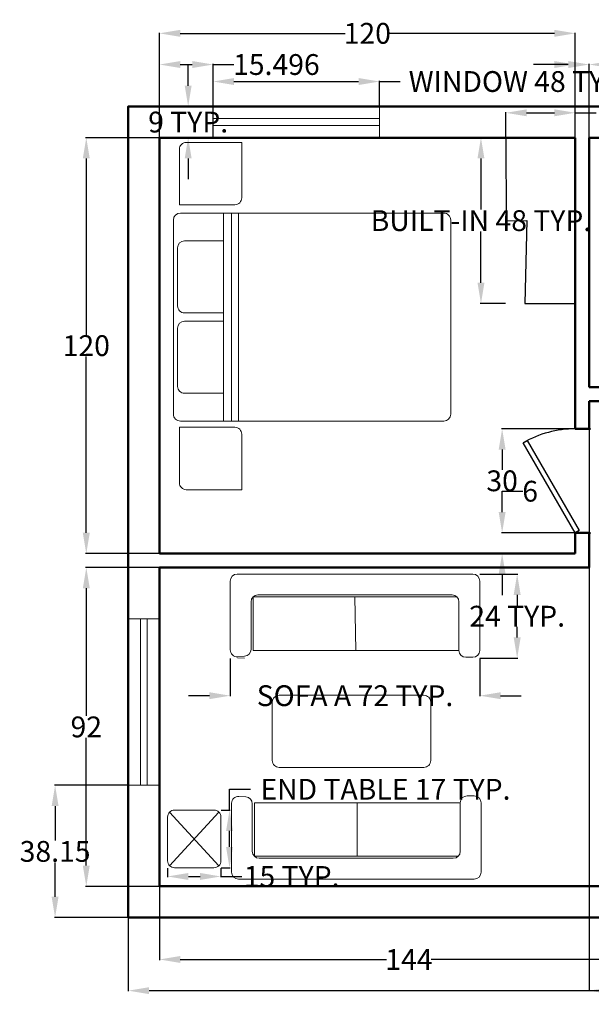
# Model space of a CAD drawing. Units: inches. Extents: x -22 to 471, y -231 to 53.
# Tile 1 of 3: x -22 to 143, y -231 to 53. Entities that reach past the tile are written whole.
import ezdxf

# ---------------------------------------------------------------- set-up
doc = ezdxf.new("R2010")
doc.units = ezdxf.units.IN
doc.header["$MEASUREMENT"] = 0
for name, color, linetype, lineweight in [('A-ANNO-DIMS', 2, 'Continuous', 18), ('A-DOOR', 3, 'Continuous', 25), ('A-FLOR-CASE', 32, 'Continuous', 25), ('A-FURN', 8, 'Continuous', 18), ('A-GLAZ', 4, 'Continuous', 18), ('A-WALL', 7, 'Continuous', 50)]:
    doc.layers.add(name, color=color, linetype=linetype, lineweight=lineweight)
doc.styles.get("Standard").update_dxf_attribs({"font": 'arial.ttf'})
doc.dimstyles.get("Standard").update_dxf_attribs({"dimtxt": 6, "dimasz": 6, "dimexe": 0.18, "dimexo": 0.0625, "dimgap": 0.09, "dimtad": 0, "dimtih": 1, "dimtoh": 1, "dimdec": 0, "dimzin": 0, "dimdsep": 46, "dimlunit": 4, "dimtxsty": 'Standard', "dimcen": 0.09, "dimadec": 0, "dimazin": 0, "dimtfac": 1, "dimtdec": 0, "dimtofl": 0, "dimtmove": 0, "dimatfit": 3, "dimfxl": 1, "dimtolj": 1, "dimtzin": 0, "dimarcsym": 0})

# ---------------------------------------------------------------- blocks, each defined once
blk = doc.blocks.new('Bed - Queen')
for p, q in [((2, 0), (58, 0)), ((0, -78), (0, -2)), ((10, -1.2), (26.8, -1.2)), ((33.2, -1.2), (50, -1.2)), ((60, -2), (60, -78)), ((8, -14.4), (8, -3.2)), ((28.8, -3.2), (28.8, -14.4)), ((31.2, -14.4), (31.2, -3.2)), ((52, -3.2), (52, -14.4)), ((0, -14.4), (60, -14.4)), ((60, -16.8), (0, -16.8)), ((60, -18.8), (0, -18.8)), ((58, -80), (2, -80))]:
    blk.add_line(p, q)
for points in [[(-17.8, -1.72), (-1.8, -1.72), (-1.8, -17.72, -0.414214), (-3.8, -19.72), (-19.8, -19.72), (-19.8, -3.72, -0.414214)], [(62.41, -1.72), (78.41, -1.72, -0.414214), (80.41, -3.72), (80.41, -19.72), (64.41, -19.72, -0.414214), (62.41, -17.72)]]:
    blk.add_lwpolyline(points, format="xyb", close=True)
for centre, start, end in [((2, -2), 90, 180), ((58, -2), 0, 90), ((10, -3.2), 90, 180), ((26.8, -3.2), 0, 90), ((33.2, -3.2), 90, 180), ((50, -3.2), 0, 90), ((2, -78), 180, 270), ((58, -78), 270, 0)]:
    blk.add_arc(centre, 2, start, end)
blk = doc.blocks.new('*U7')
for p, q in [((-40, 0), (-40, 6)), ((0, 0), (0, 6))]:
    blk.add_line(p, q)
blk.add_lwpolyline([(0, 0), (-34.64, -20), (-35.52, -18.48), (-0.87, 1.52)], close=True)
blk.add_arc((0, 0), 40, 180, 210)
blk = doc.blocks.new('WIN-48IN')
for p, q in [((0, 5.5), (48, 5.5)), ((0, 3.5), (48, 3.5))]:
    blk.add_line(p, q)
for points in [[(0, 0), (0, 9)], [(48, 9), (48, 0)]]:
    blk.add_lwpolyline(points)
blk = doc.blocks.new('SOFA-72IN-A')
for p, q in [((2, 24.28), (70, 24.28)), ((0, 2.42), (0, 22.28)), ((72, 22.28), (72, 2.28)), ((64, 18.28), (8, 18.28)), ((36.29, 2.28), (36, 17.7)), ((6, 16.28), (6, 2.56)), ((66, 2.28), (66, 16.28)), ((4.14, 0.57), (2.14, 0.43)), ((4.14, 0), (2.14, 0.14)), ((70, 0.28), (68, 0.28)), ((70, 0.28), (68, 0.28))]:
    blk.add_line(p, q)
blk.add_lwpolyline([(66, 16.28), (66, 2.28), (6.59, 2.28), (6.59, 17.7), (65.41, 17.7)])
for centre, start, end in [((2, 22.28), 90, 180), ((70, 22.28), 0, 90), ((8, 16.28), 90, 180), ((64, 16.28), 0, 90), ((2, 2.42), 180, 273.9184), ((4, 2.56), 273.9184, 0), ((68, 2.28), 180, 270), ((70, 2.28), 270, 0)]:
    blk.add_arc(centre, 2, start, end)
blk = doc.blocks.new('SOFA-72IN-B')
for p, q in [((2.14, 23.85), (4.14, 23.72)), ((68, 24), (70, 24)), ((0, 21.86), (0, 2)), ((6, 8), (6, 21.72)), ((36.29, 22), (36.29, 6.59)), ((66, 22), (66, 8)), ((72, 2), (72, 22)), ((64, 6), (8, 6)), ((2, 0), (70, 0))]:
    blk.add_line(p, q)
blk.add_lwpolyline([(66, 8), (66, 22), (6.59, 22), (6.59, 6.59), (65.41, 6.59)])
for centre, start, end in [((2, 21.86), 86.0816, 180), ((4, 21.72), 0, 86.0816), ((68, 22), 90, 180), ((70, 22), 0, 90), ((8, 8), 180, 270), ((64, 8), 270, 0), ((2, 2), 180, 270), ((70, 2), 270, 0)]:
    blk.add_arc(centre, 2, start, end)
blk = doc.blocks.new('TABLE-COFFEE')
blk.add_lwpolyline([(2, 20.83), (43.71, 20.83, -0.414214), (45.71, 18.83), (45.71, 2, -0.414214), (43.71, 0), (2, 0, -0.414214), (0, 2), (0, 18.83, -0.414214)], format="xyb", close=True)
blk = doc.blocks.new('TABLE-END')
for p, q in [((0.56, 0.61), (14.82, 16.04)), ((0.56, 16.04), (14.82, 0.61))]:
    blk.add_line(p, q)
blk.add_lwpolyline([(2, 16.65), (13.39, 16.65, -0.414214), (15.39, 14.65), (15.39, 2, -0.414214), (13.39, 0), (2, 0, -0.414214), (0, 2), (0, 14.65, -0.414214)], format="xyb", close=True)
blk = doc.blocks.new('BEDROOM-BUILTIN')
for p, q in [((0, 47.86), (0.1, 23.86)), ((0.1, 23.86), (6.1, 23.99)), ((6.1, 23.99), (5.51, 0)), ((5.51, 0), (20.03, 0))]:
    blk.add_line(p, q)
blk = doc.blocks.new('*D17')
at = {"layer": 'A-ANNO-DIMS', "color": 0, "lineweight": -2, "transparency": 16777216}
for p, q in [((33.43, 28.07), (33.43, 35.39)), ((39.43, 35.21), (75.43, 35.21)), ((81.43, 28.07), (81.43, 35.39)), ((81.43, 35.21), (87.43, 35.21))]:
    blk.add_line(p, q, dxfattribs=at)
at = {"layer": 'A-ANNO-DIMS', "color": 0, "transparency": 16777216}
for points in [[(39.43, 36.21), (39.43, 34.21), (33.43, 35.21)], [(75.43, 36.21), (75.43, 34.21), (81.43, 35.21)]]:
    blk.add_solid(points, dxfattribs=at)
at = {"layer": 'Defpoints', "color": 0, "transparency": 16777216}
for p in [(81.43, 35.21), (33.43, 28.01), (81.43, 28.01)]:
    blk.add_point(p, dxfattribs=at)
at = {"layer": 'A-ANNO-DIMS', "color": 0, "transparency": 16777216, "insert": (121.8, 35.21), "char_height": 6, "attachment_point": 5}
blk.add_mtext('\\A1;WINDOW 48 TYP.', dxfattribs=at)
blk = doc.blocks.new('*D18')
at = {"layer": 'A-ANNO-DIMS', "color": 0, "lineweight": -2, "transparency": 16777216}
for p, q in [((26.23, 34.01), (26.23, 40.01)), ((33.37, 28.01), (26.05, 28.01)), ((33.37, 19.01), (26.05, 19.01)), ((26.23, 13.01), (26.23, 7.01))]:
    blk.add_line(p, q, dxfattribs=at)
at = {"layer": 'A-ANNO-DIMS', "color": 0, "transparency": 16777216}
for points in [[(25.23, 34.01), (27.23, 34.01), (26.23, 28.01)], [(25.23, 13.01), (27.23, 13.01), (26.23, 19.01)]]:
    blk.add_solid(points, dxfattribs=at)
at = {"layer": 'Defpoints', "color": 0, "transparency": 16777216}
for p in [(26.23, 28.01), (33.43, 28.01), (33.43, 19.01)]:
    blk.add_point(p, dxfattribs=at)
at = {"layer": 'A-ANNO-DIMS', "color": 0, "transparency": 16777216, "insert": (26.23, 23.51), "char_height": 6, "attachment_point": 5}
blk.add_mtext('\\A1;9 TYP.', dxfattribs=at)
blk = doc.blocks.new('*D31')
at = {"layer": 'A-ANNO-DIMS', "color": 0, "lineweight": -2, "transparency": 16777216}
for p, q in [((38.37, -131.25), (38.37, -142.17)), ((110.37, -131.25), (110.37, -142.17)), ((32.37, -141.99), (26.37, -141.99)), ((116.37, -141.99), (122.37, -141.99))]:
    blk.add_line(p, q, dxfattribs=at)
at = {"layer": 'A-ANNO-DIMS', "color": 0, "transparency": 16777216}
for points in [[(32.37, -140.99), (32.37, -142.99), (38.37, -141.99)], [(116.37, -140.99), (116.37, -142.99), (110.37, -141.99)]]:
    blk.add_solid(points, dxfattribs=at)
at = {"layer": 'Defpoints', "color": 0, "transparency": 16777216}
for p in [(38.37, -131.19), (110.37, -131.19), (110.37, -141.99)]:
    blk.add_point(p, dxfattribs=at)
at = {"layer": 'A-ANNO-DIMS', "color": 0, "transparency": 16777216, "insert": (74.37, -141.99), "char_height": 6, "attachment_point": 5}
blk.add_mtext('\\A1;SOFA A 72 TYP.', dxfattribs=at)
blk = doc.blocks.new('*D32')
at = {"layer": 'A-ANNO-DIMS', "color": 0, "lineweight": -2, "transparency": 16777216}
for p, q in [((110.43, -106.9), (121.35, -106.9)), ((121.17, -112.9), (121.17, -115.94)), ((121.17, -125.19), (121.17, -122.15)), ((110.43, -131.19), (121.35, -131.19))]:
    blk.add_line(p, q, dxfattribs=at)
at = {"layer": 'A-ANNO-DIMS', "color": 0, "transparency": 16777216}
for points in [[(120.17, -112.9), (122.17, -112.9), (121.17, -106.9)], [(120.17, -125.19), (122.17, -125.19), (121.17, -131.19)]]:
    blk.add_solid(points, dxfattribs=at)
at = {"layer": 'Defpoints', "color": 0, "transparency": 16777216}
for p in [(110.37, -106.9), (121.17, -106.9), (110.37, -131.19)]:
    blk.add_point(p, dxfattribs=at)
at = {"layer": 'A-ANNO-DIMS', "color": 0, "transparency": 16777216, "insert": (121.17, -119.05), "char_height": 6, "attachment_point": 5}
blk.add_mtext('\\A1;24 TYP.', dxfattribs=at)
blk = doc.blocks.new('*D37')
at = {"layer": 'A-ANNO-DIMS', "color": 0, "lineweight": -2, "transparency": 16777216}
for p, q in [((38.17, -174.99), (38.17, -168.99)), ((38.17, -168.99), (44.17, -168.99)), ((35.74, -174.99), (38.35, -174.99)), ((38.17, -185.64), (38.17, -180.99)), ((35.74, -191.64), (38.35, -191.64))]:
    blk.add_line(p, q, dxfattribs=at)
at = {"layer": 'A-ANNO-DIMS', "color": 0, "transparency": 16777216}
for points in [[(37.17, -180.99), (39.17, -180.99), (38.17, -174.99)], [(37.17, -185.64), (39.17, -185.64), (38.17, -191.64)]]:
    blk.add_solid(points, dxfattribs=at)
at = {"layer": 'Defpoints', "color": 0, "transparency": 16777216}
for p in [(35.68, -174.99), (38.17, -174.99), (35.68, -191.64)]:
    blk.add_point(p, dxfattribs=at)
at = {"layer": 'A-ANNO-DIMS', "color": 0, "transparency": 16777216, "insert": (83.16, -168.99), "char_height": 6, "attachment_point": 5}
blk.add_mtext('\\A1;END TABLE 17 TYP.', dxfattribs=at)
blk = doc.blocks.new('*D38')
at = {"layer": 'A-ANNO-DIMS', "color": 0, "lineweight": -2, "transparency": 16777216}
for p, q in [((20.29, -191.7), (20.29, -194.32)), ((35.68, -191.7), (35.68, -194.32)), ((26.29, -194.14), (29.68, -194.14)), ((35.68, -194.14), (41.68, -194.14))]:
    blk.add_line(p, q, dxfattribs=at)
at = {"layer": 'A-ANNO-DIMS', "color": 0, "transparency": 16777216}
for points in [[(26.29, -193.14), (26.29, -195.14), (20.29, -194.14)], [(29.68, -193.14), (29.68, -195.14), (35.68, -194.14)]]:
    blk.add_solid(points, dxfattribs=at)
at = {"layer": 'Defpoints', "color": 0, "transparency": 16777216}
for p in [(20.29, -191.64), (35.68, -191.64), (35.68, -194.14)]:
    blk.add_point(p, dxfattribs=at)
at = {"layer": 'A-ANNO-DIMS', "color": 0, "transparency": 16777216, "insert": (56.09, -194.14), "char_height": 6, "attachment_point": 5}
blk.add_mtext('\\A1;15 TYP.', dxfattribs=at)
blk = doc.blocks.new('*D39')
at = {"layer": 'A-ANNO-DIMS', "color": 0, "lineweight": -2, "transparency": 16777216}
for p, q in [((117.84, 19.01), (110.54, 19.01)), ((110.72, 13.01), (110.72, -1.76)), ((110.72, -22.85), (110.72, -8.07)), ((117.84, -28.85), (110.54, -28.85))]:
    blk.add_line(p, q, dxfattribs=at)
at = {"layer": 'A-ANNO-DIMS', "color": 0, "transparency": 16777216}
for points in [[(109.72, 13.01), (111.72, 13.01), (110.72, 19.01)], [(109.72, -22.85), (111.72, -22.85), (110.72, -28.85)]]:
    blk.add_solid(points, dxfattribs=at)
at = {"layer": 'Defpoints', "color": 0, "transparency": 16777216}
for p in [(110.72, 19.01), (117.9, 19.01), (117.9, -28.85)]:
    blk.add_point(p, dxfattribs=at)
at = {"layer": 'A-ANNO-DIMS', "color": 0, "transparency": 16777216, "insert": (110.72, -4.92), "char_height": 6, "attachment_point": 5}
blk.add_mtext('\\A1;BUILT-IN 48 TYP.', dxfattribs=at)
blk = doc.blocks.new('*D40')
at = {"layer": 'A-ANNO-DIMS', "color": 0, "lineweight": -2, "transparency": 16777216}
for p, q in [((117.9, 19.07), (117.9, 26.37)), ((123.9, 26.19), (131.93, 26.19)), ((137.93, 19.07), (137.93, 26.37)), ((137.93, 26.19), (143.93, 26.19))]:
    blk.add_line(p, q, dxfattribs=at)
at = {"layer": 'A-ANNO-DIMS', "color": 0, "transparency": 16777216}
for points in [[(123.9, 27.19), (123.9, 25.19), (117.9, 26.19)], [(131.93, 27.19), (131.93, 25.19), (137.93, 26.19)]]:
    blk.add_solid(points, dxfattribs=at)
at = {"layer": 'Defpoints', "color": 0, "transparency": 16777216}
for p in [(137.93, 26.19), (117.9, 19.01), (137.93, 19.01)]:
    blk.add_point(p, dxfattribs=at)
at = {"layer": 'A-ANNO-DIMS', "color": 0, "transparency": 16777216, "insert": (158.68, 26.19), "char_height": 6, "attachment_point": 5}
blk.add_mtext('\\A1;20 TYP.', dxfattribs=at)
blk = doc.blocks.new('*D43')
at = {"layer": 'A-ANNO-DIMS', "color": 0, "lineweight": -2, "transparency": 16777216}
for p, q in [((8.93, -206.05), (8.93, -227.27)), ((410.93, -206.05), (410.93, -227.27)), ((14.93, -227.09), (203.13, -227.09)), ((404.93, -227.09), (216.74, -227.09))]:
    blk.add_line(p, q, dxfattribs=at)
at = {"layer": 'A-ANNO-DIMS', "color": 0, "transparency": 16777216}
for points in [[(14.93, -226.09), (14.93, -228.09), (8.93, -227.09)], [(404.93, -226.09), (404.93, -228.09), (410.93, -227.09)]]:
    blk.add_solid(points, dxfattribs=at)
at = {"layer": 'Defpoints', "color": 0, "transparency": 16777216}
for p in [(8.93, -205.99), (410.93, -205.99), (410.93, -227.09)]:
    blk.add_point(p, dxfattribs=at)
at = {"layer": 'A-ANNO-DIMS', "color": 0, "transparency": 16777216, "insert": (209.93, -227.09), "char_height": 6, "attachment_point": 5}
blk.add_mtext('\\A1;402', dxfattribs=at)
blk = doc.blocks.new('*D45')
at = {"layer": 'A-ANNO-DIMS', "color": 0, "lineweight": -2, "transparency": 16777216}
for p, q in [((17.93, 19.07), (17.93, 40.29)), ((23.93, 40.11), (27.43, 40.11)), ((33.43, 19.07), (33.43, 40.29)), ((33.43, 40.11), (39.43, 40.11))]:
    blk.add_line(p, q, dxfattribs=at)
at = {"layer": 'A-ANNO-DIMS', "color": 0, "transparency": 16777216}
for points in [[(23.93, 41.11), (23.93, 39.11), (17.93, 40.11)], [(27.43, 41.11), (27.43, 39.11), (33.43, 40.11)]]:
    blk.add_solid(points, dxfattribs=at)
at = {"layer": 'Defpoints', "color": 0, "transparency": 16777216}
for p in [(33.43, 40.11), (17.93, 19.01), (33.43, 19.01)]:
    blk.add_point(p, dxfattribs=at)
at = {"layer": 'A-ANNO-DIMS', "color": 0, "transparency": 16777216, "insert": (51.69, 40.11), "char_height": 6, "attachment_point": 5}
blk.add_mtext('\\A1;15.496', dxfattribs=at)
blk = doc.blocks.new('*D46')
at = {"layer": 'A-ANNO-DIMS', "color": 0, "lineweight": -2, "transparency": 16777216}
for p, q in [((135.93, 40.11), (129.93, 40.11)), ((141.93, 19.07), (141.93, 40.29)), ((149.06, 19.07), (149.06, 40.29)), ((155.06, 40.11), (161.06, 40.11))]:
    blk.add_line(p, q, dxfattribs=at)
at = {"layer": 'A-ANNO-DIMS', "color": 0, "transparency": 16777216}
for points in [[(135.93, 41.11), (135.93, 39.11), (141.93, 40.11)], [(155.06, 41.11), (155.06, 39.11), (149.06, 40.11)]]:
    blk.add_solid(points, dxfattribs=at)
at = {"layer": 'Defpoints', "color": 0, "transparency": 16777216}
for p in [(149.06, 40.11), (141.93, 19.01), (149.06, 19.01)]:
    blk.add_point(p, dxfattribs=at)
at = {"layer": 'A-ANNO-DIMS', "color": 0, "transparency": 16777216, "insert": (171.25, 40.11), "char_height": 6, "attachment_point": 5}
blk.add_mtext('\\A1;7.127', dxfattribs=at)
blk = doc.blocks.new('*D49')
at = {"layer": 'A-ANNO-DIMS', "color": 0, "lineweight": -2, "transparency": 16777216}
for p, q in [((17.93, -197.05), (17.93, -218.27)), ((161.93, -197.05), (161.93, -218.27)), ((23.93, -218.09), (83.51, -218.09)), ((155.93, -218.09), (96.36, -218.09))]:
    blk.add_line(p, q, dxfattribs=at)
at = {"layer": 'A-ANNO-DIMS', "color": 0, "transparency": 16777216}
for points in [[(23.93, -217.09), (23.93, -219.09), (17.93, -218.09)], [(155.93, -217.09), (155.93, -219.09), (161.93, -218.09)]]:
    blk.add_solid(points, dxfattribs=at)
at = {"layer": 'Defpoints', "color": 0, "transparency": 16777216}
for p in [(17.93, -196.99), (161.93, -196.99), (17.93, -218.09)]:
    blk.add_point(p, dxfattribs=at)
at = {"layer": 'A-ANNO-DIMS', "color": 0, "transparency": 16777216, "insert": (89.93, -218.09), "char_height": 6, "attachment_point": 5}
blk.add_mtext('\\A1;144', dxfattribs=at)
blk = doc.blocks.new('*D52')
at = {"layer": 'A-ANNO-DIMS', "color": 0, "lineweight": -2, "transparency": 16777216}
for p, q in [((17.93, 19.07), (17.93, 49.29)), ((23.93, 49.11), (71.51, 49.11)), ((131.93, 49.11), (84.36, 49.11)), ((137.93, 19.07), (137.93, 49.29))]:
    blk.add_line(p, q, dxfattribs=at)
at = {"layer": 'A-ANNO-DIMS', "color": 0, "transparency": 16777216}
for points in [[(23.93, 50.11), (23.93, 48.11), (17.93, 49.11)], [(131.93, 50.11), (131.93, 48.11), (137.93, 49.11)]]:
    blk.add_solid(points, dxfattribs=at)
at = {"layer": 'Defpoints', "color": 0, "transparency": 16777216}
for p in [(137.93, 49.11), (17.93, 19.01), (137.93, 19.01)]:
    blk.add_point(p, dxfattribs=at)
at = {"layer": 'A-ANNO-DIMS', "color": 0, "transparency": 16777216, "insert": (77.93, 49.11), "char_height": 6, "attachment_point": 5}
blk.add_mtext('\\A1;120', dxfattribs=at)
blk = doc.blocks.new('*D53')
at = {"layer": 'A-ANNO-DIMS', "color": 0, "lineweight": -2, "transparency": 16777216}
for p, q in [((17.87, 19.01), (-3.35, 19.01)), ((-3.17, 13.01), (-3.17, -37.84)), ((-3.17, -94.99), (-3.17, -44.14)), ((17.87, -100.99), (-3.35, -100.99))]:
    blk.add_line(p, q, dxfattribs=at)
at = {"layer": 'A-ANNO-DIMS', "color": 0, "transparency": 16777216}
for points in [[(-4.17, 13.01), (-2.17, 13.01), (-3.17, 19.01)], [(-4.17, -94.99), (-2.17, -94.99), (-3.17, -100.99)]]:
    blk.add_solid(points, dxfattribs=at)
at = {"layer": 'Defpoints', "color": 0, "transparency": 16777216}
for p in [(-3.17, 19.01), (17.93, 19.01), (17.93, -100.99)]:
    blk.add_point(p, dxfattribs=at)
at = {"layer": 'A-ANNO-DIMS', "color": 0, "transparency": 16777216, "insert": (-3.17, -40.99), "char_height": 6, "attachment_point": 5}
blk.add_mtext('\\A1;120', dxfattribs=at)
blk = doc.blocks.new('*D54')
at = {"layer": 'A-ANNO-DIMS', "color": 0, "lineweight": -2, "transparency": 16777216}
for p, q in [((131.93, 40.11), (125.93, 40.11)), ((137.93, 19.07), (137.93, 40.29)), ((141.93, 19.07), (141.93, 40.29)), ((147.93, 40.11), (153.93, 40.11))]:
    blk.add_line(p, q, dxfattribs=at)
at = {"layer": 'A-ANNO-DIMS', "color": 0, "transparency": 16777216}
for points in [[(131.93, 41.11), (131.93, 39.11), (137.93, 40.11)], [(147.93, 41.11), (147.93, 39.11), (141.93, 40.11)]]:
    blk.add_solid(points, dxfattribs=at)
at = {"layer": 'Defpoints', "color": 0, "transparency": 16777216}
for p in [(141.93, 40.11), (137.93, 19.01), (141.93, 19.01)]:
    blk.add_point(p, dxfattribs=at)
at = {"layer": 'A-ANNO-DIMS', "color": 0, "transparency": 16777216, "insert": (156.1, 40.11), "char_height": 6, "attachment_point": 5}
blk.add_mtext('\\A1;4', dxfattribs=at)
blk = doc.blocks.new('*D57')
at = {"layer": 'A-ANNO-DIMS', "color": 0, "lineweight": -2, "transparency": 16777216}
for p, q in [((8.87, -167.84), (-12.35, -167.84)), ((-12.17, -173.84), (-12.17, -183.76)), ((-12.17, -199.99), (-12.17, -190.07)), ((8.87, -205.99), (-12.35, -205.99))]:
    blk.add_line(p, q, dxfattribs=at)
at = {"layer": 'A-ANNO-DIMS', "color": 0, "transparency": 16777216}
for points in [[(-13.17, -173.84), (-11.17, -173.84), (-12.17, -167.84)], [(-13.17, -199.99), (-11.17, -199.99), (-12.17, -205.99)]]:
    blk.add_solid(points, dxfattribs=at)
at = {"layer": 'Defpoints', "color": 0, "transparency": 16777216}
for p in [(-12.17, -167.84), (8.93, -167.84), (8.93, -205.99)]:
    blk.add_point(p, dxfattribs=at)
at = {"layer": 'A-ANNO-DIMS', "color": 0, "transparency": 16777216, "insert": (-12.17, -186.91), "char_height": 6, "attachment_point": 5}
blk.add_mtext('\\A1;38.15', dxfattribs=at)
blk = doc.blocks.new('*D59')
at = {"layer": 'A-ANNO-DIMS', "color": 0, "lineweight": -2, "transparency": 16777216}
for p, q in [((17.87, -104.99), (-3.35, -104.99)), ((-3.17, -110.99), (-3.17, -147.84)), ((-3.17, -190.99), (-3.17, -154.14)), ((17.87, -196.99), (-3.35, -196.99))]:
    blk.add_line(p, q, dxfattribs=at)
at = {"layer": 'A-ANNO-DIMS', "color": 0, "transparency": 16777216}
for points in [[(-4.17, -110.99), (-2.17, -110.99), (-3.17, -104.99)], [(-4.17, -190.99), (-2.17, -190.99), (-3.17, -196.99)]]:
    blk.add_solid(points, dxfattribs=at)
at = {"layer": 'Defpoints', "color": 0, "transparency": 16777216}
for p in [(-3.17, -104.99), (17.93, -104.99), (17.93, -196.99)]:
    blk.add_point(p, dxfattribs=at)
at = {"layer": 'A-ANNO-DIMS', "color": 0, "transparency": 16777216, "insert": (-3.17, -150.99), "char_height": 6, "attachment_point": 5}
blk.add_mtext('\\A1;92', dxfattribs=at)
blk = doc.blocks.new('*D60')
at = {"layer": 'A-ANNO-DIMS', "color": 0, "lineweight": -2, "transparency": 16777216}
for p, q in [((137.87, -64.99), (116.65, -64.99)), ((116.83, -70.99), (116.83, -76.83)), ((116.83, -88.99), (116.83, -83.14)), ((137.87, -94.99), (116.65, -94.99))]:
    blk.add_line(p, q, dxfattribs=at)
at = {"layer": 'A-ANNO-DIMS', "color": 0, "transparency": 16777216}
for points in [[(115.83, -70.99), (117.83, -70.99), (116.83, -64.99)], [(115.83, -88.99), (117.83, -88.99), (116.83, -94.99)]]:
    blk.add_solid(points, dxfattribs=at)
at = {"layer": 'Defpoints', "color": 0, "transparency": 16777216}
for p in [(116.83, -64.99), (137.93, -64.99), (137.93, -94.99)]:
    blk.add_point(p, dxfattribs=at)
at = {"layer": 'A-ANNO-DIMS', "color": 0, "transparency": 16777216, "insert": (116.83, -79.99), "char_height": 6, "attachment_point": 5}
blk.add_mtext('\\A1;30', dxfattribs=at)
blk = doc.blocks.new('*D61')
at = {"layer": 'A-ANNO-DIMS', "color": 0, "lineweight": -2, "transparency": 16777216}
for p, q in [((116.83, -88.99), (116.83, -82.99)), ((116.83, -82.99), (122.83, -82.99)), ((137.87, -94.99), (116.65, -94.99)), ((137.87, -100.99), (116.65, -100.99)), ((116.83, -106.99), (116.83, -112.99))]:
    blk.add_line(p, q, dxfattribs=at)
at = {"layer": 'A-ANNO-DIMS', "color": 0, "transparency": 16777216}
for points in [[(115.83, -88.99), (117.83, -88.99), (116.83, -94.99)], [(115.83, -106.99), (117.83, -106.99), (116.83, -100.99)]]:
    blk.add_solid(points, dxfattribs=at)
at = {"layer": 'Defpoints', "color": 0, "transparency": 16777216}
for p in [(116.83, -94.99), (137.93, -94.99), (137.93, -100.99)]:
    blk.add_point(p, dxfattribs=at)
at = {"layer": 'A-ANNO-DIMS', "color": 0, "transparency": 16777216, "insert": (124.91, -82.99), "char_height": 6, "attachment_point": 5}
blk.add_mtext('\\A1;6', dxfattribs=at)
blk = doc.blocks.new('*D62')
at = {"layer": 'A-ANNO-DIMS', "color": 0, "lineweight": -2, "transparency": 16777216}
for p, q in [((141.93, -57.05), (141.93, -227.27)), ((162.85, -57.05), (162.85, -227.27)), ((147.93, -227.09), (156.85, -227.09)), ((162.85, -227.09), (168.85, -227.09))]:
    blk.add_line(p, q, dxfattribs=at)
at = {"layer": 'A-ANNO-DIMS', "color": 0, "transparency": 16777216}
for points in [[(147.93, -226.09), (147.93, -228.09), (141.93, -227.09)], [(156.85, -226.09), (156.85, -228.09), (162.85, -227.09)]]:
    blk.add_solid(points, dxfattribs=at)
at = {"layer": 'Defpoints', "color": 0, "transparency": 16777216}
for p in [(141.93, -56.99), (162.85, -56.99), (162.85, -227.09)]:
    blk.add_point(p, dxfattribs=at)
at = {"layer": 'A-ANNO-DIMS', "color": 0, "transparency": 16777216, "insert": (181.44, -227.09), "char_height": 6, "attachment_point": 5}
blk.add_mtext('\\A1;20.916', dxfattribs=at)

msp = doc.modelspace()

# ---------------------------------------------------------------- linework, layer by layer
at = {"layer": 'A-WALL'}
for p, q in [((17.9344, 19.0112), (137.9344, 19.0112)), ((17.9344, -100.9888), (17.9344, 19.0112)), ((137.9344, -64.9888), (137.9344, 19.0112)), ((141.9344, -52.9888), (141.9344, 19.0112)), ((141.9344, 19.0112), (205.9344, 19.0112)), ((141.9344, -52.9888), (158.4725, -52.9888)), ((141.9344, -56.9888), (162.85, -56.9888)), ((141.9344, -64.9888), (141.9344, -56.9888)), ((137.9344, -64.9888), (141.9344, -64.9888)), ((137.9344, -100.9888), (137.9344, -94.9888)), ((137.9344, -94.9888), (141.9344, -94.9888)), ((141.9344, -104.9888), (141.9344, -94.9888)), ((17.9344, -100.9888), (137.9344, -100.9888)), ((17.9344, -196.9888), (17.9344, -104.9888)), ((17.9344, -104.9888), (141.9344, -104.9888)), ((161.9344, -196.9888), (17.9344, -196.9888))]:
    msp.add_line(p, q, dxfattribs=at)
msp.add_lwpolyline([(161.9344, -205.9888), (8.9344, -205.9888), (8.9344, 28.0112), (218.9344, 28.0112)], dxfattribs=at)

# ---------------------------------------------------------------- block references
at = {"layer": 'A-DOOR', "xscale": 0.75, "yscale": 0.75, "zscale": 0.75, "rotation": 270}
msp.add_blockref('*U7', (137.9344, -94.9888), dxfattribs=at)
at = {"layer": 'A-FLOR-CASE'}
msp.add_blockref('BEDROOM-BUILTIN', (117.902, -28.845), dxfattribs=at)
at = {"layer": 'A-FURN', "rotation": 89.99999999999999}
msp.add_blockref('Bed - Queen', (21.9796, -62.7501), dxfattribs=at)
at = {"layer": 'A-FURN'}
for name, p in [('SOFA-72IN-A', (38.368, -131.187)), ('TABLE-COFFEE', (50.516, -162.683)), ('SOFA-72IN-B', (38.744, -194.884)), ('TABLE-END', (20.292, -191.641))]:
    msp.add_blockref(name, p, dxfattribs=at)
at = {"layer": 'A-GLAZ'}
msp.add_blockref('WIN-48IN', (33.4305, 19.011), dxfattribs=at)
at = {"layer": 'A-GLAZ', "rotation": 270}
msp.add_blockref('WIN-48IN', (8.9343, -119.8401), dxfattribs=at)

# ---------------------------------------------------------------- dimensions: what is measured, and where the dimension line sits
at = {"layer": 'A-ANNO-DIMS'}
for base, p1, p2, override, picture, middle in [((137.9344, 49.1112), (17.9344, 19.0112), (137.9344, 19.0112), {"dimdec": 0, "dimlfac": 1, "dimrnd": 0, "dimzin": 0, "dimdsep": 46, "dimlunit": 2}, '*D52', (77.9344, 49.1112)), ((33.4306, 40.1112), (17.9344, 19.0112), (33.4306, 19.0112), {"dimdec": 3, "dimlfac": 1, "dimrnd": 0, "dimzin": 0, "dimdsep": 46, "dimlunit": 2}, '*D45', (51.6905, 40.1112)), ((141.9344, 40.1112), (137.9344, 19.0112), (141.9344, 19.0112), {"dimdec": 0, "dimlfac": 1, "dimrnd": 0, "dimzin": 0, "dimdsep": 46, "dimlunit": 2}, '*D54', (156.0995, 40.1112)), ((162.85, -227.0888), (141.9344, -56.9888), (162.85, -56.9888), {"dimdec": 3, "dimlfac": 1, "dimrnd": 0, "dimzin": 0, "dimdsep": 46, "dimlunit": 2}, '*D62', (181.4434, -227.0888)), ((410.9344, -227.0888), (8.9344, -205.9888), (410.9344, -205.9888), {"dimdec": 0, "dimlfac": 1, "dimrnd": 0, "dimzin": 0, "dimdsep": 46, "dimlunit": 2}, '*D43', (209.9344, -227.0888))]:
    dim = msp.add_linear_dim(base=base, p1=p1, p2=p2, dimstyle='Standard', override=override, dxfattribs=at)
    dim.commit()
    dim.dimension.update_dxf_attribs({"geometry": picture, "text_midpoint": middle})
for base, p1, p2, text, picture, middle in [((81.4306, 35.2112), (33.4306, 28.0112), (81.4306, 28.0112), 'WINDOW <> TYP.', '*D17', (121.7996, 35.2112)), ((137.9344, 26.1896), (117.9021, 19.0112), (137.9344, 19.0112), '<> TYP.', '*D40', (158.6786, 26.1896)), ((110.3681, -141.9874), (38.3681, -131.1874), (110.3681, -131.1874), 'SOFA A <> TYP.', '*D31', (74.3681, -141.9874)), ((35.6773, -194.1388), (20.2916, -191.6413), (35.6773, -191.6413), '<> TYP.', '*D38', (56.0879, -194.1388))]:
    dim = msp.add_linear_dim(base=base, p1=p1, p2=p2, text=text, dimstyle='Standard', override={"dimdec": 0, "dimlfac": 1, "dimrnd": 0, "dimzin": 0, "dimdsep": 46, "dimlunit": 2}, dxfattribs=at)
    dim.commit()
    dim.dimension.update_dxf_attribs({"geometry": picture, "text_midpoint": middle})
for base, p1, p2, angle, override, picture, middle in [((149.0611, 40.1112), (141.9344, 19.0112), (149.0611, 19.0112), 0, {"dimdec": 3, "dimlfac": 1, "dimrnd": 0, "dimzin": 0, "dimdsep": 46, "dimlunit": 2}, '*D46', (171.25, 40.1112)), ((-3.1656, 19.0112), (17.9344, -100.9888), (17.9344, 19.0112), 90, {"dimdec": 0, "dimlfac": 1, "dimrnd": 0, "dimzin": 0, "dimdsep": 46, "dimlunit": 2}, '*D53', (-3.1656, -40.9888)), ((116.8344, -64.9888), (137.9344, -94.9888), (137.9344, -64.9888), 90, {"dimdec": 0, "dimlfac": 1, "dimrnd": 0, "dimzin": 0, "dimdsep": 46, "dimlunit": 2}, '*D60', (116.8344, -79.9888)), ((116.8344, -94.9888), (137.9344, -100.9888), (137.9344, -94.9888), 90, {"dimdec": 0, "dimlfac": 1, "dimrnd": 0, "dimzin": 0, "dimdsep": 46, "dimlunit": 2}, '*D61', (124.9053, -82.9888)), ((-3.1656, -104.9888), (17.9344, -196.9888), (17.9344, -104.9888), 90, {"dimdec": 0, "dimlfac": 1, "dimrnd": 0, "dimzin": 0, "dimdsep": 46, "dimlunit": 2}, '*D59', (-3.1656, -150.9888)), ((-12.1656, -167.8402), (8.9344, -205.9888), (8.9344, -167.8402), 90, {"dimdec": 2, "dimlfac": 1, "dimrnd": 0, "dimzin": 0, "dimdsep": 46, "dimlunit": 2}, '*D57', (-12.1656, -186.9145)), ((17.9344, -218.0888), (161.9344, -196.9888), (17.9344, -196.9888), 180, {"dimdec": 0, "dimlfac": 1, "dimrnd": 0, "dimzin": 0, "dimdsep": 46, "dimlunit": 2}, '*D49', (89.9344, -218.0888))]:
    dim = msp.add_linear_dim(base=base, p1=p1, p2=p2, angle=angle, dimstyle='Standard', override=override, dxfattribs=at)
    dim.commit()
    dim.dimension.update_dxf_attribs({"geometry": picture, "text_midpoint": middle})
for base, p1, p2, text, picture, middle in [((26.2306, 28.0112), (33.4306, 19.0112), (33.4306, 28.0112), '<> TYP.', '*D18', (26.2306, 23.5112)), ((110.7236, 19.0112), (117.9021, -28.845), (117.9021, 19.0112), 'BUILT-IN <> TYP.', '*D39', (110.7236, -4.9169)), ((121.1681, -106.9041), (110.3681, -131.1874), (110.3681, -106.9041), '<> TYP.', '*D32', (121.1681, -119.0458)), ((38.1748, -174.9913), (35.6773, -191.6413), (35.6773, -174.9913), 'END TABLE <> TYP.', '*D37', (83.1646, -168.9913))]:
    dim = msp.add_linear_dim(base=base, p1=p1, p2=p2, angle=90, text=text, dimstyle='Standard', override={"dimdec": 0, "dimlfac": 1, "dimrnd": 0, "dimzin": 0, "dimdsep": 46, "dimlunit": 2}, dxfattribs=at)
    dim.commit()
    dim.dimension.update_dxf_attribs({"geometry": picture, "text_midpoint": middle})

doc.saveas('drawing.dxf')
